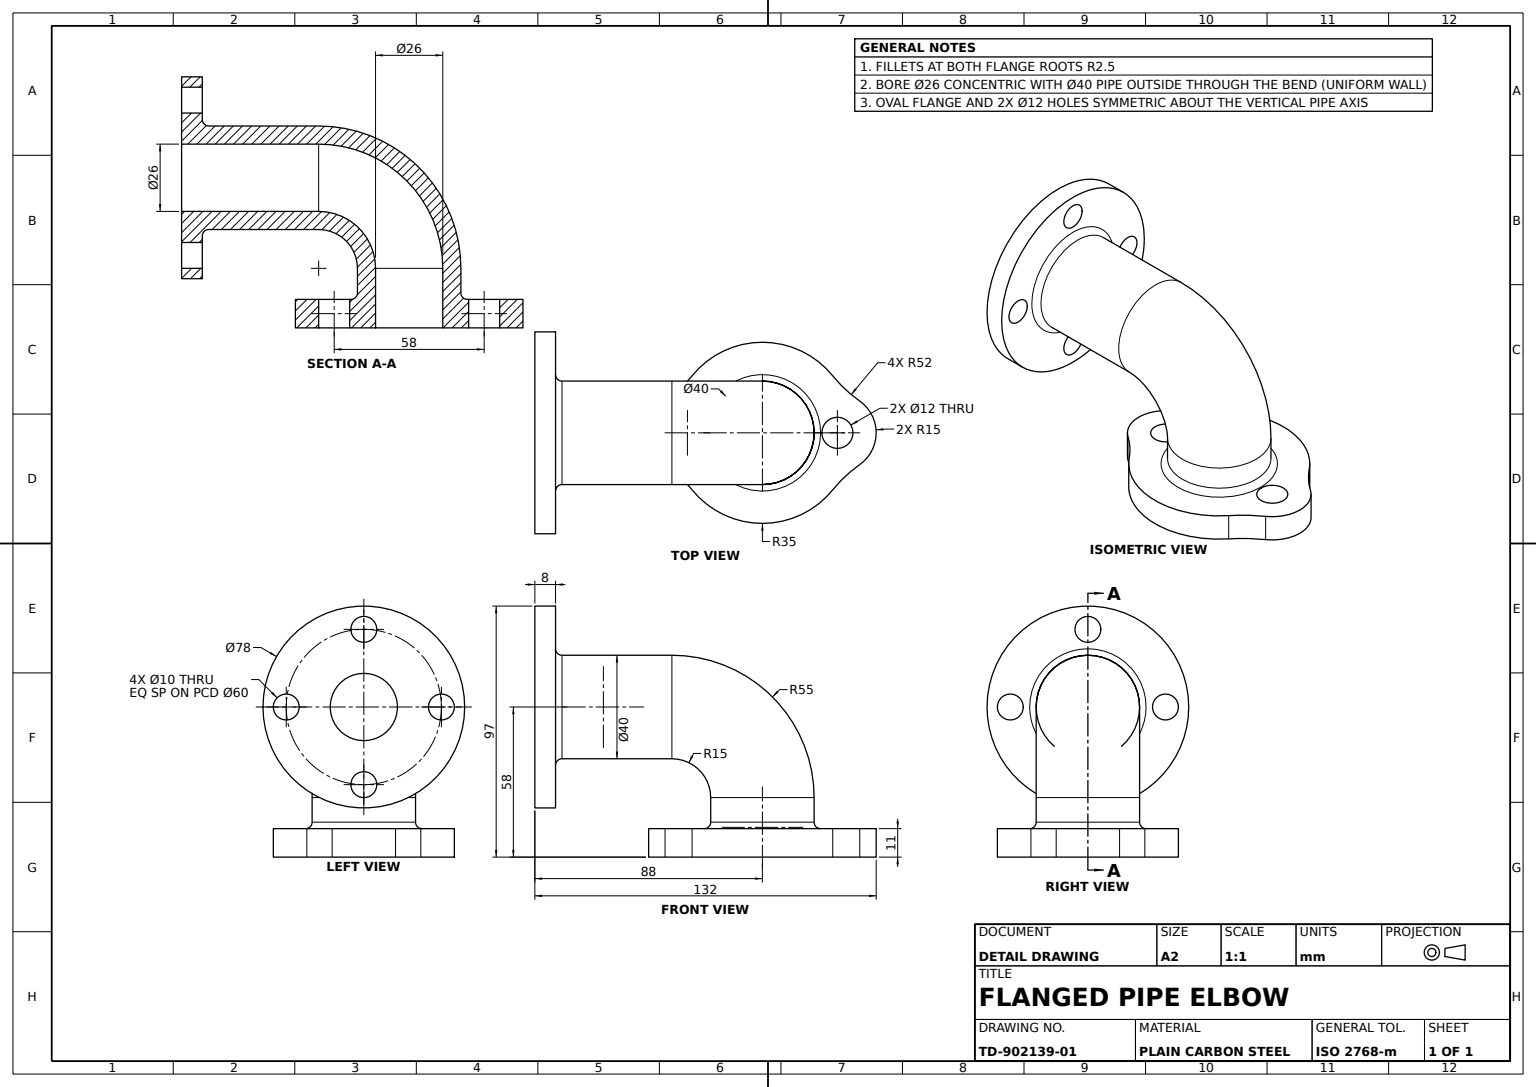
from build123d import *

# Parameters (mm, degrees)
PIPE_SECTION_SKETCH_40X_26_R        = 20
PIPE_SECTION_SKETCH_40X_26_R_2      = 13
ROUND_START                         = 8
ROUND_FLANGE_SKETCH_78_R            = 39
ROUND_FLANGE_SKETCH_78_R_2          = 13
ROUND_FLANGE_78_DEPTH               = 8
ROUND_FLANGE_BOLT_HOLES_4X_10_REACH = 130.643
ROUND_FLANGE_BOLT_HOLES_SKETCH_R    = 5
OVAL_FLANGE_SKETCH_R                = 6
OVAL_FLANGE_SKETCH_R_2              = 13
OVAL_FLANGE_DEPTH                   = 11
FLANGE_ROOT_FILLETS_R2_5_R          = 2.5


with BuildPart() as part:
    # Elbow Pipe Body: sweep along a path in Elbow Path Sketch
    with BuildLine(Plane.XY) as elbow_pipe_body_path:
        Line((0, 0), (53, 0))
        ThreePointArc((53, 0), (77.748737342, -10.251262658), (88, -35))
        Line((88, -35), (88, -58))
    # Pipe Section Sketch Ø40xØ26 → Elbow Pipe Body (sweep)
    with BuildSketch(Plane(origin=(0, 0, 0), x_dir=(0, 0, -1), z_dir=(1, 0, 0))):
        Circle(PIPE_SECTION_SKETCH_40X_26_R)
        Circle(PIPE_SECTION_SKETCH_40X_26_R_2, mode=Mode.SUBTRACT)
    sweep(path=elbow_pipe_body_path.line)

    # Round Flange Sketch Ø78 → Round Flange Ø78 (add)
    with BuildSketch(Plane(origin=(0, 0, 0), x_dir=(0, 0, -1), z_dir=(1, 0, 0)).offset(ROUND_START)):
        Circle(ROUND_FLANGE_SKETCH_78_R)
        with Locations(Location((0, 0, 0), (0, 0, 90))):
            Circle(ROUND_FLANGE_SKETCH_78_R_2, mode=Mode.SUBTRACT)
    extrude(amount=-ROUND_FLANGE_78_DEPTH)

    # Round Flange Bolt Holes Sketch → Round Flange Bolt Holes 4xØ10 (cut, up to next)
    with BuildSketch(Plane.ZY, mode=Mode.PRIVATE) as round_flange_bolt_holes_4x_10_sk1:
        with Locations((0, 30)):
            Circle(ROUND_FLANGE_BOLT_HOLES_SKETCH_R)
    round_flange_bolt_holes_4x_10_tool1 = extrude(round_flange_bolt_holes_4x_10_sk1.sketch, amount=-ROUND_FLANGE_BOLT_HOLES_4X_10_REACH, mode=Mode.PRIVATE) & part.part
    # Round Flange Bolt Holes Sketch → Round Flange Bolt Holes 4xØ10 (cut, up to next)
    with BuildSketch(Plane.ZY, mode=Mode.PRIVATE) as round_flange_bolt_holes_4x_10_sk2:
        with Locations((30, 0)):
            Circle(ROUND_FLANGE_BOLT_HOLES_SKETCH_R)
    round_flange_bolt_holes_4x_10_tool2 = extrude(round_flange_bolt_holes_4x_10_sk2.sketch, amount=-ROUND_FLANGE_BOLT_HOLES_4X_10_REACH, mode=Mode.PRIVATE) & part.part
    # Round Flange Bolt Holes Sketch → Round Flange Bolt Holes 4xØ10 (cut, up to next)
    with BuildSketch(Plane.ZY, mode=Mode.PRIVATE) as round_flange_bolt_holes_4x_10_sk3:
        with Locations((0, -30)):
            Circle(ROUND_FLANGE_BOLT_HOLES_SKETCH_R)
    round_flange_bolt_holes_4x_10_tool3 = extrude(round_flange_bolt_holes_4x_10_sk3.sketch, amount=-ROUND_FLANGE_BOLT_HOLES_4X_10_REACH, mode=Mode.PRIVATE) & part.part
    # Round Flange Bolt Holes Sketch → Round Flange Bolt Holes 4xØ10 (cut, up to next)
    with BuildSketch(Plane.ZY, mode=Mode.PRIVATE) as round_flange_bolt_holes_4x_10_sk4:
        with Locations((-30, 0)):
            Circle(ROUND_FLANGE_BOLT_HOLES_SKETCH_R)
    round_flange_bolt_holes_4x_10_tool4 = extrude(round_flange_bolt_holes_4x_10_sk4.sketch, amount=-ROUND_FLANGE_BOLT_HOLES_4X_10_REACH, mode=Mode.PRIVATE) & part.part
    add(round_flange_bolt_holes_4x_10_tool1.solids().sort_by_distance((0, 30, 0))[0], mode=Mode.SUBTRACT)
    add(round_flange_bolt_holes_4x_10_tool2.solids().sort_by_distance((0, 0, 30))[0], mode=Mode.SUBTRACT)
    add(round_flange_bolt_holes_4x_10_tool3.solids().sort_by_distance((0, -30, 0))[0], mode=Mode.SUBTRACT)
    add(round_flange_bolt_holes_4x_10_tool4.solids().sort_by_distance((0, 0, -30))[0], mode=Mode.SUBTRACT)

    # Oval Flange Sketch → Oval Flange (add)
    with BuildSketch(Plane.XZ.offset(58)):
        with BuildLine():
            ThreePointArc((60.803210464, -22.030311821), (88, -35), (115.196789536, -22.030311821))
            ThreePointArc((115.196789536, -22.030311821), (120.082146816, -16.784263387), (125.642563047, -12.259938988))
            ThreePointArc((125.642563047, -12.259938988), (132, 0), (125.642563047, 12.259938988))
            ThreePointArc((125.642563047, 12.259938988), (120.082146816, 16.784263387), (115.196789536, 22.030311821))
            ThreePointArc((115.196789536, 22.030311821), (88, 35), (60.803210464, 22.030311821))
            ThreePointArc((60.803210464, 22.030311821), (55.917853184, 16.784263387), (50.357436953, 12.259938988))
            ThreePointArc((50.357436953, 12.259938988), (44, 0), (50.357436953, -12.259938988))
            ThreePointArc((50.357436953, -12.259938988), (55.917853184, -16.784263387), (60.803210464, -22.030311821))
        make_face()
        with Locations((117, 0)):
            Circle(OVAL_FLANGE_SKETCH_R, mode=Mode.SUBTRACT)
        with Locations((59, 0)):
            Circle(OVAL_FLANGE_SKETCH_R, mode=Mode.SUBTRACT)
        with Locations(Location((88, 0, 0), (0, 0, 270))):
            Circle(OVAL_FLANGE_SKETCH_R_2, mode=Mode.SUBTRACT)
    extrude(amount=-OVAL_FLANGE_DEPTH)

    # Flange Root Fillets R2.5
    flange_root_fillets_r2_5_edges = [part.edges().sort_by_distance(p)[0] for p in [
        (8, 0, 20),
        (88, -47, 20),
    ]]
    fillet(flange_root_fillets_r2_5_edges, radius=FLANGE_ROOT_FILLETS_R2_5_R)


solid = part.part
